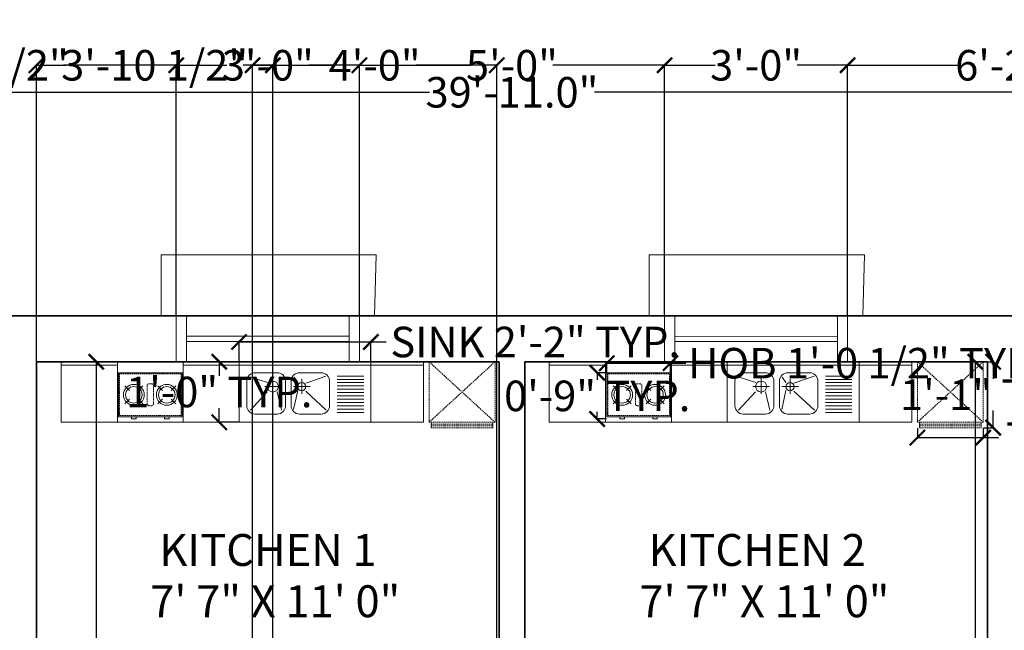
# Model space of a CAD drawing. Units: inches. Extents: x 844 to 2234, y 346 to 1084.
# Tile 45 of 93: x 1093 to 1287, y 964 to 1084. Entities that reach past the tile are written whole.
import ezdxf

# ---------------------------------------------------------------- set-up
doc = ezdxf.new("R2010")
doc.units = ezdxf.units.IN
doc.header["$MEASUREMENT"] = 0
doc.linetypes.add('HIDDEN', pattern=[0.375, 0.25, -0.125])
for name, color, linetype, lineweight in [('A-ANNO-DIMS', 2, 'Continuous', 18), ('A-AREA-IDEN', 7, 'Continuous', 18), ('A-EQPM', 42, 'Continuous', 18), ('A-EQPM-HIDN', 42, 'HIDDEN', 13), ('A-FLOR-CASE', 42, 'Continuous', 18), ('A-FLOR-FIXT', 8, 'Continuous', 18), ('A-WALL', 7, 'Continuous', 35), ('windows', 1, 'Continuous', 18)]:
    doc.layers.add(name, color=color, linetype=linetype, lineweight=lineweight)
doc.styles.get("Standard").update_dxf_attribs({"font": 'arial.ttf'})
doc.dimstyles.get("Standard").update_dxf_attribs({"dimtxt": 6, "dimasz": 3, "dimexe": 0.18, "dimexo": 0.0625, "dimgap": 0.09, "dimtad": 0, "dimtih": 1, "dimtoh": 1, "dimdec": 1, "dimzin": 0, "dimdsep": 46, "dimlunit": 3, "dimtxsty": 'Standard', "dimblk": 'ARCHTICK', "dimcen": 0.09, "dimadec": 0, "dimazin": 0, "dimtfac": 1, "dimtdec": 1, "dimtofl": 0, "dimtmove": 0, "dimatfit": 3, "dimfxl": 1, "dimtolj": 1, "dimtzin": 0, "dimarcsym": 0})

# ---------------------------------------------------------------- blocks, each defined once
blk = doc.blocks.new('_ArchTick')
at = {"color": 0, "linetype": 'ByBlock', "const_width": 0.15}
blk.add_lwpolyline([(-0.5, -0.5), (0.5, 0.5)], dxfattribs=at)
blk = doc.blocks.new('*D26')
at = {"layer": 'A-ANNO-DIMS', "color": 0, "lineweight": -2, "transparency": 16777216}
for p, q in [((1099.7, 1016.31), (1108.56, 1016.31)), ((1108.38, 1016.31), (1108.38, 953.41)), ((1108.38, 884.31), (1108.38, 947.21)), ((1099.7, 884.31), (1108.56, 884.31))]:
    blk.add_line(p, q, dxfattribs=at)
at = {"layer": 'Defpoints', "color": 0, "transparency": 16777216}
for p in [(1099.64, 1016.31), (1099.64, 884.31), (1108.38, 884.31)]:
    blk.add_point(p, dxfattribs=at)
at = {"layer": 'A-ANNO-DIMS', "color": 0, "lineweight": -2, "transparency": 16777216, "xscale": 3, "yscale": 3, "zscale": 3}
for p, rotation in [((1108.38, 1016.31), 90), ((1108.38, 884.31), 270)]:
    blk.add_blockref('_ArchTick', p, dxfattribs=dict(at, rotation=rotation))
at = {"layer": 'A-ANNO-DIMS', "color": 0, "transparency": 16777216, "insert": (1108.38, 950.31), "char_height": 6, "attachment_point": 5}
blk.add_mtext("\\A1;11'", dxfattribs=at)
blk = doc.blocks.new('*D27')
at = {"layer": 'A-ANNO-DIMS', "color": 0, "lineweight": -2, "transparency": 16777216}
for p, q in [((1283.21, 1016.31), (1281.03, 1016.31)), ((1281.21, 1016.31), (1281.21, 953.41)), ((1281.21, 884.31), (1281.21, 947.21)), ((1283.21, 884.31), (1281.03, 884.31))]:
    blk.add_line(p, q, dxfattribs=at)
at = {"layer": 'Defpoints', "color": 0, "transparency": 16777216}
for p in [(1283.27, 1016.31), (1281.21, 884.31), (1283.27, 884.31)]:
    blk.add_point(p, dxfattribs=at)
at = {"layer": 'A-ANNO-DIMS', "color": 0, "lineweight": -2, "transparency": 16777216, "xscale": 3, "yscale": 3, "zscale": 3}
for p, rotation in [((1281.21, 1016.31), 90), ((1281.21, 884.31), 270)]:
    blk.add_blockref('_ArchTick', p, dxfattribs=dict(at, rotation=rotation))
at = {"layer": 'A-ANNO-DIMS', "color": 0, "transparency": 16777216, "insert": (1281.21, 950.31), "char_height": 6, "attachment_point": 5}
blk.add_mtext("\\A1;11'", dxfattribs=at)
blk = doc.blocks.new('*D55')
at = {"layer": 'A-ANNO-DIMS', "color": 0, "lineweight": -2, "transparency": 16777216}
for p, q in [((950.62, 1025.37), (950.62, 1069.43)), ((950.62, 1069.25), (1173.9, 1069.25)), ((1429.62, 1069.25), (1206.34, 1069.25)), ((1429.62, 1025.37), (1429.62, 1069.43))]:
    blk.add_line(p, q, dxfattribs=at)
at = {"layer": 'Defpoints', "color": 0, "transparency": 16777216}
for p in [(1429.62, 1069.25), (950.62, 1025.31), (1429.62, 1025.31)]:
    blk.add_point(p, dxfattribs=at)
at = {"layer": 'A-ANNO-DIMS', "color": 0, "lineweight": -2, "transparency": 16777216, "xscale": 3, "yscale": 3, "zscale": 3, "rotation": 180}
blk.add_blockref('_ArchTick', (950.62, 1069.25), dxfattribs=at)
at = {"layer": 'A-ANNO-DIMS', "color": 0, "lineweight": -2, "transparency": 16777216, "xscale": 3, "yscale": 3, "zscale": 3}
blk.add_blockref('_ArchTick', (1429.62, 1069.25), dxfattribs=at)
at = {"layer": 'A-ANNO-DIMS', "color": 0, "transparency": 16777216, "insert": (1190.12, 1069.25), "char_height": 6, "attachment_point": 5}
blk.add_mtext('\\A1;39\'-11.0"', dxfattribs=at)
blk = doc.blocks.new('WIN-36IN')
for p, q in [((0, 9), (0, 21)), ((0, 21), (42.29, 21)), ((42, 9), (42.29, 21)), ((3, 9), (0, 9)), ((39, 9), (3, 9)), ((3, 9), (3, 0)), ((5, 9), (5, 0)), ((37, 0), (37, 9)), ((39, 0), (39, 9)), ((39, 9), (42, 9)), ((5, 5), (37, 5)), ((5, 4), (37, 4)), ((3, 0), (39, 0))]:
    blk.add_line(p, q)
blk = doc.blocks.new('KITCHEN-TALL-UNIT')
for p, q in [((12.96, 1.08), (0, 12.96)), ((0, 1.08), (12.96, 12.96)), ((0.43, 0.73), (12.53, 0.73)), ((0.43, 0.37), (12.53, 0.37))]:
    blk.add_line(p, q)
blk.add_lwpolyline([(0, 1.08), (0, 12.96), (12.96, 12.96), (12.96, 1.08)], close=True)
blk.add_lwpolyline([(0.43, 1.08), (0.43, 0), (12.53, 0), (12.53, 1.08)])
blk = doc.blocks.new('KITCHEN-COUNTER-LINEAR')
for p, q in [((0, 11.88), (34.99, 11.88)), ((0, 11.88), (0, 0)), ((11.08, 11.88), (11.08, 0)), ((24.04, 11.88), (24.04, 0)), ((60.91, 11.88), (71.28, 11.88)), ((71.28, 11.88), (71.28, 0)), ((0, 11.23), (11.08, 11.23)), ((24.04, 11.23), (34.99, 11.23)), ((34.99, 11.23), (60.91, 11.23)), ((60.91, 11.23), (71.28, 11.23)), ((0, 0), (34.99, 0)), ((60.91, 0), (71.28, 0))]:
    blk.add_line(p, q)
blk = doc.blocks.new('HOB-2-BURNER')
for p, q in [((1.27, 6.49), (2.18, 5.57)), ((3.86, 5.57), (4.78, 6.49)), ((7.75, 6.49), (8.66, 5.57)), ((10.34, 5.57), (11.26, 6.49)), ((1.27, 2.97), (2.18, 3.89)), ((3.86, 3.89), (4.78, 2.97)), ((7.75, 2.97), (8.66, 3.89)), ((10.34, 3.89), (11.26, 2.97))]:
    blk.add_line(p, q)
blk.add_lwpolyline([(0, 9.07), (0, 0.43), (12.53, 0.43), (12.53, 9.07)], close=True)
for points in [[(2.59, 0.43), (2.59, 0), (3.46, 0), (3.46, 0.45)], [(9.07, 0.43), (9.07, 0), (9.94, 0), (9.94, 0.45)]]:
    blk.add_lwpolyline(points)
for centre, radius in [((3.02, 4.73), 2.05), ((3.02, 4.73), 1.62), ((9.5, 4.73), 2.05), ((9.5, 4.73), 1.62)]:
    blk.add_circle(centre, radius)
blk = doc.blocks.new('SINK-DOUBLE-DRAINBOARD')
for p, q in [((5.62, 7.84), (2.31, 8.86)), ((6.65, 5.57), (6.65, 8.58)), ((11.53, 7.78), (10.82, 8.86)), ((12.33, 5.55), (12.33, 8.55)), ((13.11, 7.71), (17.09, 9.07)), ((19.31, 9.07), (24.52, 9.07)), ((19.31, 8.42), (24.52, 8.42)), ((19.31, 7.78), (24.52, 7.78)), ((2.23, 2.35), (5.55, 5.96)), ((5.05, 7.02), (8.29, 7.02)), ((8.36, 2.35), (7.5, 5.96)), ((10.74, 7), (13.98, 7)), ((11.53, 6.26), (10.74, 2.51)), ((13.11, 6.11), (17.15, 2.35)), ((19.31, 7.13), (24.52, 7.13)), ((19.31, 6.48), (24.52, 6.48)), ((19.31, 5.83), (24.52, 5.83)), ((19.31, 5.18), (24.52, 5.18)), ((19.31, 4.54), (24.52, 4.54)), ((19.31, 3.89), (24.52, 3.89)), ((19.31, 3.24), (24.52, 3.24)), ((19.31, 2.59), (24.52, 2.59)), ((19.31, 1.94), (24.52, 1.94))]:
    blk.add_line(p, q)
blk.add_lwpolyline([(0, 0), (25.92, 0), (25.92, 11.88), (0, 11.88)], close=True)
for points in [[(1.51, 8.1), (1.51, 3.24, 0.414214), (3.13, 1.62), (7.54, 1.62, 0.414214), (9.16, 3.24), (9.16, 8.1, 0.414214), (7.54, 9.72), (3.13, 9.72, 0.414214)], [(10.24, 8.1), (10.24, 3.24, 0.414214), (11.86, 1.62), (16.18, 1.62, 0.414214), (17.8, 3.24), (17.8, 8.1, 0.414214), (16.18, 9.72), (11.86, 9.72, 0.414214)]]:
    blk.add_lwpolyline(points, format="xyb", close=True)
for centre, radius in [((6.65, 7.02), 1.08), ((12.33, 7), 0.81)]:
    blk.add_circle(centre, radius)
blk = doc.blocks.new('*D125')
at = {"layer": 'A-ANNO-DIMS', "color": 0, "lineweight": -2, "transparency": 16777216}
for p, q in [((1269.83, 1003.29), (1269.83, 1001.23)), ((1282.79, 1003.29), (1282.79, 1001.23)), ((1269.83, 1001.41), (1282.79, 1001.41)), ((1282.79, 1001.41), (1285.79, 1001.41))]:
    blk.add_line(p, q, dxfattribs=at)
at = {"layer": 'Defpoints', "color": 0, "transparency": 16777216}
for p in [(1269.83, 1003.35), (1282.79, 1003.35), (1282.79, 1001.41)]:
    blk.add_point(p, dxfattribs=at)
at = {"layer": 'A-ANNO-DIMS', "color": 0, "lineweight": -2, "transparency": 16777216, "xscale": 3, "yscale": 3, "zscale": 3, "rotation": 180}
blk.add_blockref('_ArchTick', (1269.83, 1001.41), dxfattribs=at)
at = {"layer": 'A-ANNO-DIMS', "color": 0, "lineweight": -2, "transparency": 16777216, "xscale": 3, "yscale": 3, "zscale": 3}
blk.add_blockref('_ArchTick', (1282.79, 1001.41), dxfattribs=at)
at = {"layer": 'A-ANNO-DIMS', "color": 0, "transparency": 16777216, "insert": (1326.36, 1001.41), "char_height": 6, "attachment_point": 5}
blk.add_mtext('\\A1;TALL UNIT 1\'-1" TYP.', dxfattribs=at)
blk = doc.blocks.new('*D126')
at = {"layer": 'A-ANNO-DIMS', "color": 0, "lineweight": -2, "transparency": 16777216}
for p, q in [((1282.85, 1016.31), (1284.91, 1016.31)), ((1284.73, 1016.31), (1284.73, 1012.93)), ((1284.73, 1003.35), (1284.73, 1006.73)), ((1282.85, 1003.35), (1284.91, 1003.35))]:
    blk.add_line(p, q, dxfattribs=at)
at = {"layer": 'Defpoints', "color": 0, "transparency": 16777216}
for p in [(1282.79, 1016.31), (1284.73, 1016.31), (1282.79, 1003.35)]:
    blk.add_point(p, dxfattribs=at)
at = {"layer": 'A-ANNO-DIMS', "color": 0, "lineweight": -2, "transparency": 16777216, "xscale": 3, "yscale": 3, "zscale": 3}
for p, rotation in [((1284.73, 1016.31), 90), ((1284.73, 1003.35), 270)]:
    blk.add_blockref('_ArchTick', p, dxfattribs=dict(at, rotation=rotation))
at = {"layer": 'A-ANNO-DIMS', "color": 0, "transparency": 16777216, "insert": (1284.73, 1009.83), "char_height": 6, "attachment_point": 5}
blk.add_mtext('\\A1;1\'-1" TYP.', dxfattribs=at)
blk = doc.blocks.new('*D133')
at = {"layer": 'A-ANNO-DIMS', "color": 0, "lineweight": -2, "transparency": 16777216}
for p, q in [((1208.76, 1014.21), (1208.76, 1016.21)), ((1208.76, 1016.03), (1221.29, 1016.03)), ((1221.29, 1014.21), (1221.29, 1016.21)), ((1221.29, 1016.03), (1224.29, 1016.03))]:
    blk.add_line(p, q, dxfattribs=at)
at = {"layer": 'Defpoints', "color": 0, "transparency": 16777216}
for p in [(1221.29, 1016.03), (1208.76, 1014.15), (1221.29, 1014.15)]:
    blk.add_point(p, dxfattribs=at)
at = {"layer": 'A-ANNO-DIMS', "color": 0, "lineweight": -2, "transparency": 16777216, "xscale": 3, "yscale": 3, "zscale": 3, "rotation": 180}
blk.add_blockref('_ArchTick', (1208.76, 1016.03), dxfattribs=at)
at = {"layer": 'A-ANNO-DIMS', "color": 0, "lineweight": -2, "transparency": 16777216, "xscale": 3, "yscale": 3, "zscale": 3}
blk.add_blockref('_ArchTick', (1221.29, 1016.03), dxfattribs=at)
at = {"layer": 'A-ANNO-DIMS', "color": 0, "transparency": 16777216, "insert": (1259.74, 1016.03), "char_height": 6, "attachment_point": 5}
blk.add_mtext('\\A1;HOB 1\'-0 1/2" TYP.', dxfattribs=at)
blk = doc.blocks.new('*D134')
at = {"layer": 'A-ANNO-DIMS', "color": 0, "lineweight": -2, "transparency": 16777216}
for p, q in [((1208.7, 1014.15), (1206.7, 1014.15)), ((1206.88, 1014.15), (1206.88, 1012.77)), ((1208.7, 1005.08), (1206.7, 1005.08)), ((1206.88, 1005.08), (1206.88, 1006.46))]:
    blk.add_line(p, q, dxfattribs=at)
at = {"layer": 'Defpoints', "color": 0, "transparency": 16777216}
for p in [(1206.88, 1014.15), (1208.76, 1014.15), (1208.76, 1005.08)]:
    blk.add_point(p, dxfattribs=at)
at = {"layer": 'A-ANNO-DIMS', "color": 0, "lineweight": -2, "transparency": 16777216, "xscale": 3, "yscale": 3, "zscale": 3}
for p, rotation in [((1206.88, 1014.15), 90), ((1206.88, 1005.08), 270)]:
    blk.add_blockref('_ArchTick', p, dxfattribs=dict(at, rotation=rotation))
at = {"layer": 'A-ANNO-DIMS', "color": 0, "transparency": 16777216, "insert": (1206.88, 1009.61), "char_height": 6, "attachment_point": 5}
blk.add_mtext('\\A1;0\'-9" TYP.', dxfattribs=at)
blk = doc.blocks.new('*D137')
at = {"layer": 'A-ANNO-DIMS', "color": 0, "lineweight": -2, "transparency": 16777216}
for p, q in [((1136.46, 1016.37), (1136.46, 1020.38)), ((1162.38, 1016.37), (1162.38, 1020.38)), ((1136.46, 1020.2), (1162.38, 1020.2)), ((1162.38, 1020.2), (1165.38, 1020.2))]:
    blk.add_line(p, q, dxfattribs=at)
at = {"layer": 'Defpoints', "color": 0, "transparency": 16777216}
for p in [(1162.38, 1020.2), (1136.46, 1016.31), (1162.38, 1016.31)]:
    blk.add_point(p, dxfattribs=at)
at = {"layer": 'A-ANNO-DIMS', "color": 0, "lineweight": -2, "transparency": 16777216, "xscale": 3, "yscale": 3, "zscale": 3, "rotation": 180}
blk.add_blockref('_ArchTick', (1136.46, 1020.2), dxfattribs=at)
at = {"layer": 'A-ANNO-DIMS', "color": 0, "lineweight": -2, "transparency": 16777216, "xscale": 3, "yscale": 3, "zscale": 3}
blk.add_blockref('_ArchTick', (1162.38, 1020.2), dxfattribs=at)
at = {"layer": 'A-ANNO-DIMS', "color": 0, "transparency": 16777216, "insert": (1194.69, 1020.2), "char_height": 6, "attachment_point": 5}
blk.add_mtext('\\A1;SINK 2\'-2" TYP.', dxfattribs=at)
blk = doc.blocks.new('*D138')
at = {"layer": 'A-ANNO-DIMS', "color": 0, "lineweight": -2, "transparency": 16777216}
for p, q in [((1136.4, 1016.31), (1132.39, 1016.31)), ((1132.57, 1016.31), (1132.57, 1013.52)), ((1132.57, 1004.43), (1132.57, 1007.22)), ((1136.4, 1004.43), (1132.39, 1004.43))]:
    blk.add_line(p, q, dxfattribs=at)
at = {"layer": 'Defpoints', "color": 0, "transparency": 16777216}
for p in [(1132.57, 1016.31), (1136.46, 1016.31), (1136.46, 1004.43)]:
    blk.add_point(p, dxfattribs=at)
at = {"layer": 'A-ANNO-DIMS', "color": 0, "lineweight": -2, "transparency": 16777216, "xscale": 3, "yscale": 3, "zscale": 3}
for p, rotation in [((1132.57, 1016.31), 90), ((1132.57, 1004.43), 270)]:
    blk.add_blockref('_ArchTick', p, dxfattribs=dict(at, rotation=rotation))
at = {"layer": 'A-ANNO-DIMS', "color": 0, "transparency": 16777216, "insert": (1132.57, 1010.37), "char_height": 6, "attachment_point": 5}
blk.add_mtext('\\A1;1\'-0" TYP.', dxfattribs=at)
blk = doc.blocks.new('*D143')
at = {"layer": 'A-ANNO-DIMS', "color": 0, "lineweight": -2, "transparency": 16777216}
for p, q in [((1139.12, 430.37), (1139.12, 1074.74)), ((1139.12, 1074.56), (1154.93, 1074.56)), ((1187.12, 1074.56), (1171.3, 1074.56)), ((1187.12, 430.37), (1187.12, 1074.74))]:
    blk.add_line(p, q, dxfattribs=at)
at = {"layer": 'Defpoints', "color": 0, "transparency": 16777216}
for p in [(1187.12, 1074.56), (1139.12, 430.31), (1187.12, 430.31)]:
    blk.add_point(p, dxfattribs=at)
at = {"layer": 'A-ANNO-DIMS', "color": 0, "lineweight": -2, "transparency": 16777216, "xscale": 3, "yscale": 3, "zscale": 3, "rotation": 180}
blk.add_blockref('_ArchTick', (1139.12, 1074.56), dxfattribs=at)
at = {"layer": 'A-ANNO-DIMS', "color": 0, "lineweight": -2, "transparency": 16777216, "xscale": 3, "yscale": 3, "zscale": 3}
blk.add_blockref('_ArchTick', (1187.12, 1074.56), dxfattribs=at)
at = {"layer": 'A-ANNO-DIMS', "color": 0, "transparency": 16777216, "insert": (1163.12, 1074.56), "char_height": 6, "attachment_point": 5}
blk.add_mtext('\\A1;4\'-0"', dxfattribs=at)
blk = doc.blocks.new('*D144')
at = {"layer": 'A-ANNO-DIMS', "color": 0, "lineweight": -2, "transparency": 16777216}
for p, q in [((1096.62, 439.37), (1096.62, 1074.74)), ((1096.62, 1074.56), (1102.48, 1074.56)), ((1143.12, 1074.56), (1137.25, 1074.56)), ((1143.12, 492.37), (1143.12, 1074.74))]:
    blk.add_line(p, q, dxfattribs=at)
at = {"layer": 'Defpoints', "color": 0, "transparency": 16777216}
for p in [(1143.12, 1074.56), (1143.12, 492.31), (1096.62, 439.31)]:
    blk.add_point(p, dxfattribs=at)
at = {"layer": 'A-ANNO-DIMS', "color": 0, "lineweight": -2, "transparency": 16777216, "xscale": 3, "yscale": 3, "zscale": 3, "rotation": 180}
blk.add_blockref('_ArchTick', (1096.62, 1074.56), dxfattribs=at)
at = {"layer": 'A-ANNO-DIMS', "color": 0, "lineweight": -2, "transparency": 16777216, "xscale": 3, "yscale": 3, "zscale": 3}
blk.add_blockref('_ArchTick', (1143.12, 1074.56), dxfattribs=at)
at = {"layer": 'A-ANNO-DIMS', "color": 0, "transparency": 16777216, "insert": (1119.87, 1074.56), "char_height": 6, "attachment_point": 5}
blk.add_mtext('\\A1;3\'-10 1/2"', dxfattribs=at)
blk = doc.blocks.new('*D152')
at = {"layer": 'A-ANNO-DIMS', "color": 0, "lineweight": -2, "transparency": 16777216}
for p, q in [((1049.62, 1025.37), (1049.62, 1074.74)), ((1049.62, 1074.56), (1071.79, 1074.56)), ((1124.12, 1074.56), (1101.94, 1074.56)), ((1124.12, 1025.37), (1124.12, 1074.74))]:
    blk.add_line(p, q, dxfattribs=at)
at = {"layer": 'Defpoints', "color": 0, "transparency": 16777216}
for p in [(1124.12, 1074.56), (1049.62, 1025.31), (1124.12, 1025.31)]:
    blk.add_point(p, dxfattribs=at)
at = {"layer": 'A-ANNO-DIMS', "color": 0, "lineweight": -2, "transparency": 16777216, "xscale": 3, "yscale": 3, "zscale": 3, "rotation": 180}
blk.add_blockref('_ArchTick', (1049.62, 1074.56), dxfattribs=at)
at = {"layer": 'A-ANNO-DIMS', "color": 0, "lineweight": -2, "transparency": 16777216, "xscale": 3, "yscale": 3, "zscale": 3}
blk.add_blockref('_ArchTick', (1124.12, 1074.56), dxfattribs=at)
at = {"layer": 'A-ANNO-DIMS', "color": 0, "transparency": 16777216, "insert": (1086.87, 1074.56), "char_height": 6, "attachment_point": 5}
blk.add_mtext('\\A1;6\'-2 1/2"', dxfattribs=at)
blk = doc.blocks.new('*D153')
at = {"layer": 'A-ANNO-DIMS', "color": 0, "lineweight": -2, "transparency": 16777216}
for p, q in [((1124.12, 1025.37), (1124.12, 1074.74)), ((1124.12, 1074.56), (1134.05, 1074.56)), ((1160.12, 1074.56), (1150.18, 1074.56)), ((1160.12, 1025.37), (1160.12, 1074.74))]:
    blk.add_line(p, q, dxfattribs=at)
at = {"layer": 'Defpoints', "color": 0, "transparency": 16777216}
for p in [(1160.12, 1074.56), (1124.12, 1025.31), (1160.12, 1025.31)]:
    blk.add_point(p, dxfattribs=at)
at = {"layer": 'A-ANNO-DIMS', "color": 0, "lineweight": -2, "transparency": 16777216, "xscale": 3, "yscale": 3, "zscale": 3, "rotation": 180}
blk.add_blockref('_ArchTick', (1124.12, 1074.56), dxfattribs=at)
at = {"layer": 'A-ANNO-DIMS', "color": 0, "lineweight": -2, "transparency": 16777216, "xscale": 3, "yscale": 3, "zscale": 3}
blk.add_blockref('_ArchTick', (1160.12, 1074.56), dxfattribs=at)
at = {"layer": 'A-ANNO-DIMS', "color": 0, "transparency": 16777216, "insert": (1142.12, 1074.56), "char_height": 6, "attachment_point": 5}
blk.add_mtext('\\A1;3\'-0"', dxfattribs=at)
blk = doc.blocks.new('*D154')
at = {"layer": 'A-ANNO-DIMS', "color": 0, "lineweight": -2, "transparency": 16777216}
for p, q in [((1160.12, 1025.37), (1160.12, 1074.74)), ((1160.12, 1074.56), (1182.05, 1074.56)), ((1220.12, 1074.56), (1198.18, 1074.56)), ((1220.12, 1025.38), (1220.12, 1074.74))]:
    blk.add_line(p, q, dxfattribs=at)
at = {"layer": 'Defpoints', "color": 0, "transparency": 16777216}
for p in [(1220.12, 1074.56), (1160.12, 1025.31), (1220.12, 1025.31)]:
    blk.add_point(p, dxfattribs=at)
at = {"layer": 'A-ANNO-DIMS', "color": 0, "lineweight": -2, "transparency": 16777216, "xscale": 3, "yscale": 3, "zscale": 3, "rotation": 180}
blk.add_blockref('_ArchTick', (1160.12, 1074.56), dxfattribs=at)
at = {"layer": 'A-ANNO-DIMS', "color": 0, "lineweight": -2, "transparency": 16777216, "xscale": 3, "yscale": 3, "zscale": 3}
blk.add_blockref('_ArchTick', (1220.12, 1074.56), dxfattribs=at)
at = {"layer": 'A-ANNO-DIMS', "color": 0, "transparency": 16777216, "insert": (1190.12, 1074.56), "char_height": 6, "attachment_point": 5}
blk.add_mtext('\\A1;5\'-0"', dxfattribs=at)
blk = doc.blocks.new('*D155')
at = {"layer": 'A-ANNO-DIMS', "color": 0, "lineweight": -2, "transparency": 16777216}
for p, q in [((1220.12, 1025.38), (1220.12, 1074.74)), ((1220.12, 1074.56), (1230.05, 1074.56)), ((1256.12, 1074.56), (1246.18, 1074.56)), ((1256.12, 1025.37), (1256.12, 1074.74))]:
    blk.add_line(p, q, dxfattribs=at)
at = {"layer": 'Defpoints', "color": 0, "transparency": 16777216}
for p in [(1256.12, 1074.56), (1220.12, 1025.31), (1256.12, 1025.31)]:
    blk.add_point(p, dxfattribs=at)
at = {"layer": 'A-ANNO-DIMS', "color": 0, "lineweight": -2, "transparency": 16777216, "xscale": 3, "yscale": 3, "zscale": 3, "rotation": 180}
blk.add_blockref('_ArchTick', (1220.12, 1074.56), dxfattribs=at)
at = {"layer": 'A-ANNO-DIMS', "color": 0, "lineweight": -2, "transparency": 16777216, "xscale": 3, "yscale": 3, "zscale": 3}
blk.add_blockref('_ArchTick', (1256.12, 1074.56), dxfattribs=at)
at = {"layer": 'A-ANNO-DIMS', "color": 0, "transparency": 16777216, "insert": (1238.12, 1074.56), "char_height": 6, "attachment_point": 5}
blk.add_mtext('\\A1;3\'-0"', dxfattribs=at)
blk = doc.blocks.new('*D156')
at = {"layer": 'A-ANNO-DIMS', "color": 0, "lineweight": -2, "transparency": 16777216}
for p, q in [((1256.12, 1025.37), (1256.12, 1074.74)), ((1256.12, 1074.56), (1278.29, 1074.56)), ((1330.62, 1074.56), (1308.44, 1074.56)), ((1330.62, 1025.37), (1330.62, 1074.74))]:
    blk.add_line(p, q, dxfattribs=at)
at = {"layer": 'Defpoints', "color": 0, "transparency": 16777216}
for p in [(1330.62, 1074.56), (1256.12, 1025.31), (1330.62, 1025.31)]:
    blk.add_point(p, dxfattribs=at)
at = {"layer": 'A-ANNO-DIMS', "color": 0, "lineweight": -2, "transparency": 16777216, "xscale": 3, "yscale": 3, "zscale": 3, "rotation": 180}
blk.add_blockref('_ArchTick', (1256.12, 1074.56), dxfattribs=at)
at = {"layer": 'A-ANNO-DIMS', "color": 0, "lineweight": -2, "transparency": 16777216, "xscale": 3, "yscale": 3, "zscale": 3}
blk.add_blockref('_ArchTick', (1330.62, 1074.56), dxfattribs=at)
at = {"layer": 'A-ANNO-DIMS', "color": 0, "transparency": 16777216, "insert": (1293.37, 1074.56), "char_height": 6, "attachment_point": 5}
blk.add_mtext('\\A1;6\'-2 1/2"', dxfattribs=at)

msp = doc.modelspace()

# ---------------------------------------------------------------- linework, layer by layer
at = {"layer": 'A-EQPM-HIDN'}
for points in [[(1112.98, 1013.93), (1112.98, 1005.73), (1125.07, 1005.73), (1125.07, 1013.93)], [(1208.98, 1013.93), (1208.98, 1005.73), (1221.07, 1005.73), (1221.07, 1013.93)]]:
    msp.add_lwpolyline(points, close=True, dxfattribs=at)
for points in [[(1118.38, 1011.56), (1118.38, 1008.1, 0.414214), (1118.81, 1007.67), (1119.24, 1007.67, 0.414214), (1119.67, 1008.1), (1119.67, 1011.56, 0.414214), (1119.24, 1011.99), (1118.81, 1011.99, 0.414214)], [(1214.38, 1011.56), (1214.38, 1008.1, 0.414214), (1214.81, 1007.67), (1215.24, 1007.67, 0.414214), (1215.67, 1008.1), (1215.67, 1011.56, 0.414214), (1215.24, 1011.99), (1214.81, 1011.99, 0.414214)]]:
    msp.add_lwpolyline(points, format="xyb", close=True, dxfattribs=at)
at = {"layer": 'A-FLOR-FIXT'}
for p, q in [((1238.07, 1012.27), (1234.77, 1013.29)), ((1239.11, 1010), (1239.11, 1013.01)), ((1243.99, 1012.21), (1243.28, 1013.29)), ((1244.79, 1009.98), (1244.79, 1012.98)), ((1245.57, 1012.14), (1249.54, 1013.5)), ((1251.77, 1013.5), (1256.97, 1013.5)), ((1251.77, 1012.85), (1256.97, 1012.85)), ((1237.51, 1011.45), (1240.75, 1011.45)), ((1243.19, 1011.43), (1246.43, 1011.43)), ((1243.99, 1010.69), (1243.19, 1006.94)), ((1245.57, 1010.54), (1249.61, 1006.78)), ((1251.77, 1012.21), (1256.97, 1012.21)), ((1251.77, 1011.56), (1256.97, 1011.56)), ((1251.77, 1010.91), (1256.97, 1010.91)), ((1234.68, 1006.78), (1238.01, 1010.39)), ((1240.82, 1006.78), (1239.95, 1010.39)), ((1251.77, 1010.26), (1256.97, 1010.26)), ((1251.77, 1009.61), (1256.97, 1009.61)), ((1251.77, 1008.97), (1256.97, 1008.97)), ((1251.77, 1008.32), (1256.97, 1008.32)), ((1251.77, 1007.67), (1256.97, 1007.67)), ((1251.77, 1007.02), (1256.97, 1007.02)), ((1251.77, 1006.37), (1256.97, 1006.37))]:
    msp.add_line(p, q, dxfattribs=at)
msp.add_lwpolyline([(1232.46, 1004.43), (1258.38, 1004.43), (1258.38, 1016.31), (1232.46, 1016.31)], close=True, dxfattribs=at)
for points in [[(1233.97, 1012.53), (1233.97, 1007.67, 0.414214), (1235.59, 1006.05), (1240, 1006.05, 0.414214), (1241.62, 1007.67), (1241.62, 1012.53, 0.414214), (1240, 1014.15), (1235.59, 1014.15, 0.414214)], [(1242.7, 1012.53), (1242.7, 1007.67, 0.414214), (1244.32, 1006.05), (1248.64, 1006.05, 0.414214), (1250.26, 1007.67), (1250.26, 1012.53, 0.414214), (1248.64, 1014.15), (1244.32, 1014.15, 0.414214)]]:
    msp.add_lwpolyline(points, format="xyb", close=True, dxfattribs=at)
for centre, radius in [((1239.11, 1011.45), 1.08), ((1244.79, 1011.43), 0.81)]:
    msp.add_circle(centre, radius, dxfattribs=at)
at = {"layer": 'A-WALL'}
for p, q in [((950.62, 1025.31), (1429.62, 1025.31)), ((1096.62, 1016.31), (1096.62, 884.31)), ((1096.62, 1016.31), (1187.62, 1016.31)), ((1187.62, 1016.31), (1187.62, 884.31)), ((1192.62, 1016.31), (1192.62, 884.31)), ((1192.62, 1016.31), (1283.62, 1016.31)), ((1283.62, 1016.31), (1283.62, 884.31))]:
    msp.add_line(p, q, dxfattribs=at)

# ---------------------------------------------------------------- block references
at = {"layer": 'A-EQPM'}
for p in [(1112.76, 1005.08), (1208.76, 1005.08)]:
    msp.add_blockref('HOB-2-BURNER', p, dxfattribs=at)
at = {"layer": 'A-EQPM-HIDN'}
for p in [(1173.83, 1003.35), (1269.83, 1003.35)]:
    msp.add_blockref('KITCHEN-TALL-UNIT', p, dxfattribs=at)
at = {"layer": 'A-FLOR-CASE'}
for p in [(1101.46, 1004.43), (1197.46, 1004.43)]:
    msp.add_blockref('KITCHEN-COUNTER-LINEAR', p, dxfattribs=at)
at = {"layer": 'A-FLOR-FIXT'}
msp.add_blockref('SINK-DOUBLE-DRAINBOARD', (1136.46, 1004.43), dxfattribs=at)
at = {"layer": 'windows'}
msp.add_blockref('WIN-36IN', (1121.12, 1016.31), dxfattribs=at)
at = {"layer": 'windows', "rotation": 359.9931124012453}
msp.add_blockref('WIN-36IN', (1217.12, 1016.31), dxfattribs=at)

# ---------------------------------------------------------------- texts
at = {"layer": 'A-AREA-IDEN'}
for s, height, p in [('KITCHEN 1', 6.269, (1120.79, 976.2)), ('KITCHEN 2', 6.269, (1216.96, 976.2)), (' 7\' 7" X 11\' 0"', 6.2688, (1117.09, 966.13)), (' 7\' 7" X 11\' 0"', 6.2688, (1213.26, 966.13))]:
    msp.add_text(s, height=height, dxfattribs=at).set_placement(p)

# ---------------------------------------------------------------- dimensions: what is measured, and where the dimension line sits
at = {"layer": 'A-ANNO-DIMS'}
for base, p1, p2, override, picture, middle in [((1124.12, 1074.56), (1049.62, 1025.31), (1124.12, 1025.31), {"dimdec": 1, "dimlfac": 1, "dimrnd": 0, "dimzin": 1, "dimdsep": 46, "dimlunit": 4, "dimfrac": 2}, '*D152', (1086.87, 1074.56)), ((1143.12, 1074.56), (1096.62, 439.31), (1143.12, 492.31), {"dimdec": 1, "dimlfac": 1, "dimrnd": 0, "dimzin": 1, "dimdsep": 46, "dimlunit": 4, "dimfrac": 2}, '*D144', (1119.87, 1074.56)), ((1330.62, 1074.56), (1256.12, 1025.31), (1330.62, 1025.31), {"dimdec": 1, "dimlfac": 1, "dimrnd": 0, "dimzin": 1, "dimdsep": 46, "dimlunit": 4, "dimfrac": 2}, '*D156', (1293.37, 1074.56)), ((1160.12, 1074.56), (1124.12, 1025.31), (1160.12, 1025.31), {"dimdec": 1, "dimlfac": 1, "dimrnd": 0, "dimzin": 1, "dimdsep": 46, "dimlunit": 4, "dimfrac": 2}, '*D153', (1142.12, 1074.56)), ((1187.12, 1074.56), (1139.12, 430.31), (1187.12, 430.31), {"dimdec": 1, "dimlfac": 1, "dimrnd": 0, "dimzin": 1, "dimdsep": 46, "dimlunit": 4, "dimfrac": 2}, '*D143', (1163.12, 1074.56)), ((1220.12, 1074.56), (1160.12, 1025.31), (1220.12, 1025.31), {"dimdec": 1, "dimlfac": 1, "dimrnd": 0, "dimzin": 1, "dimdsep": 46, "dimlunit": 4, "dimfrac": 2}, '*D154', (1190.12, 1074.56)), ((1256.12, 1074.56), (1220.12, 1025.31), (1256.12, 1025.31), {"dimdec": 1, "dimlfac": 1, "dimrnd": 0, "dimzin": 1, "dimdsep": 46, "dimlunit": 4, "dimfrac": 2}, '*D155', (1238.12, 1074.56)), ((1429.62, 1069.25), (950.62, 1025.31), (1429.62, 1025.31), {"dimclrd": 0, "dimclre": 0, "dimclrt": 0}, '*D55', (1190.12, 1069.25))]:
    dim = msp.add_linear_dim(base=base, p1=p1, p2=p2, dimstyle='Standard', override=override, dxfattribs=at)
    dim.commit()
    dim.dimension.update_dxf_attribs({"geometry": picture, "text_midpoint": middle})
for base, p1, p2, text, picture, middle in [((1162.38, 1020.2), (1136.46, 1016.31), (1162.38, 1016.31), 'SINK <> TYP.', '*D137', (1194.69, 1020.2)), ((1221.29, 1016.03), (1208.76, 1014.15), (1221.29, 1014.15), 'HOB <> TYP.', '*D133', (1259.74, 1016.03)), ((1282.79, 1001.41), (1269.83, 1003.35), (1282.79, 1003.35), 'TALL UNIT <> TYP.', '*D125', (1326.36, 1001.41))]:
    dim = msp.add_linear_dim(base=base, p1=p1, p2=p2, text=text, dimstyle='Standard', override={"dimdec": 1, "dimlfac": 1, "dimrnd": 0, "dimzin": 1, "dimdsep": 46, "dimlunit": 4, "dimfrac": 2}, dxfattribs=at)
    dim.commit()
    dim.dimension.update_dxf_attribs({"geometry": picture, "text_midpoint": middle})
for base, p1, p2, picture, middle in [((1132.57, 1016.31), (1136.46, 1004.43), (1136.46, 1016.31), '*D138', (1132.57, 1010.37)), ((1206.88, 1014.15), (1208.76, 1005.08), (1208.76, 1014.15), '*D134', (1206.88, 1009.61)), ((1284.73, 1016.31), (1282.79, 1003.35), (1282.79, 1016.31), '*D126', (1284.73, 1009.83))]:
    dim = msp.add_linear_dim(base=base, p1=p1, p2=p2, angle=90, text='<> TYP.', dimstyle='Standard', override={"dimdec": 1, "dimlfac": 1, "dimrnd": 0, "dimzin": 1, "dimdsep": 46, "dimlunit": 4, "dimfrac": 2}, dxfattribs=at)
    dim.commit()
    dim.dimension.update_dxf_attribs({"geometry": picture, "text_midpoint": middle})
for base, p1, p2, picture, middle in [((1108.38, 884.31), (1099.64, 1016.31), (1099.64, 884.31), '*D26', (1108.38, 950.31)), ((1281.21, 884.31), (1283.27, 1016.31), (1283.27, 884.31), '*D27', (1281.21, 950.31))]:
    dim = msp.add_linear_dim(base=base, p1=p1, p2=p2, angle=90, dimstyle='Standard', override={"dimclrd": 0, "dimclre": 0, "dimclrt": 0}, dxfattribs=at)
    dim.commit()
    dim.dimension.update_dxf_attribs({"geometry": picture, "text_midpoint": middle})

doc.saveas('drawing.dxf')
